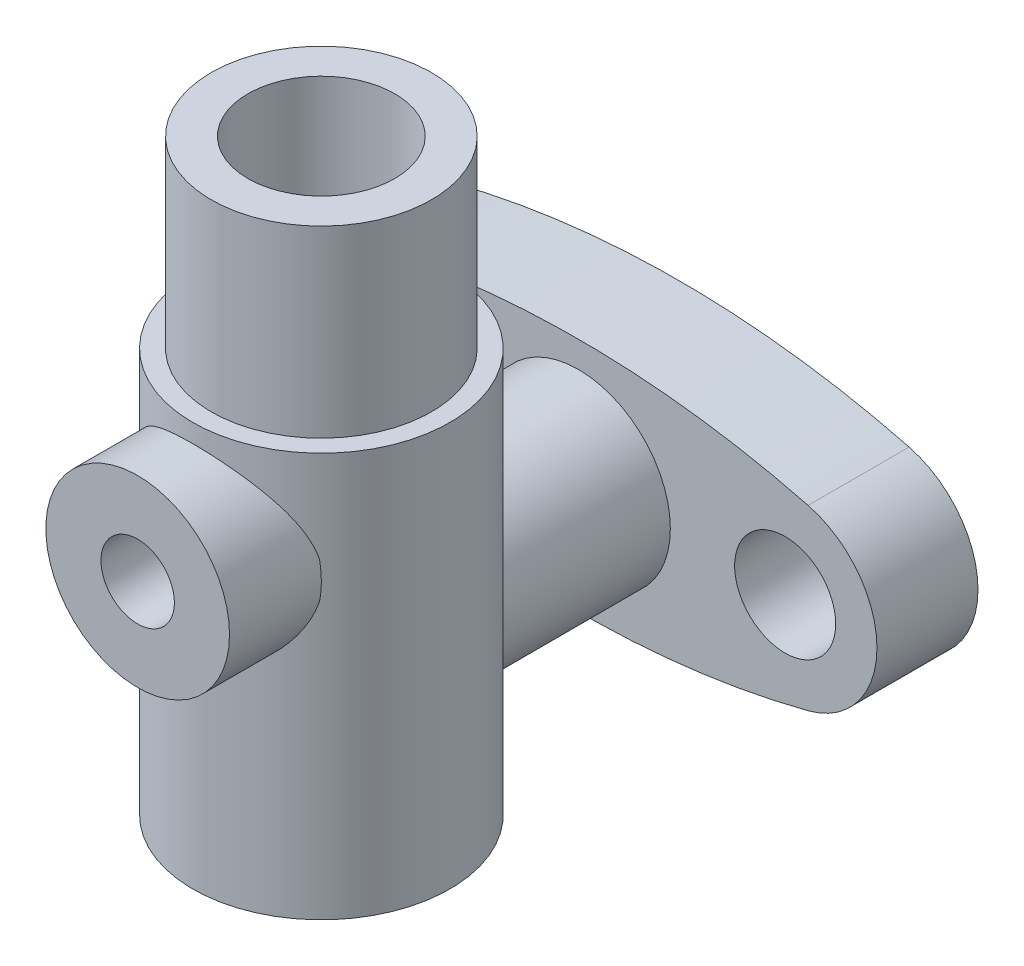
SolidWorks part; units mm, degrees
material "Plain Carbon Steel"
ref_plane "Front Plane" through (0, 0, 0) normal (0, 0, 1) x (1, 0, 0)
ref_plane "Top Plane" through (0, 0, 0) normal (0, 1, 0) x (1, 0, 0)
ref_plane "Right Plane" through (0, 0, 0) normal (1, 0, 0) x (0, 0, -1)
sketch "Main Body Profile Sketch" plane through (0, 0, 0) normal (0, 0, 1) x (1, 0, 0)
  line L0 (0, 64) -> (0, 0) construction
  line L1 (0, 64) -> (12, 64)
  line L2 (12, 64) -> (12, 44)
  line L3 (12, 44) -> (14, 44)
  line L4 (14, 44) -> (14, 0)
  line L5 (14, 0) -> (0, 0)
  line L6 (0, 0) -> (0, 64)
  dimension "D1" = 24
  dimension "D2" = 28
  dimension "D3" = 64
  dimension "D4" = 44
revolve "Main Body Revolve" add sketch "Main Body Profile Sketch" angle 360 about L0
cosmetic thread "Cosmetic Thread1" parameters "D1"=19, "D2"=13.797
ref_plane "Plane1" through (0, 0, 20) normal (0, 0, 1) x (1, 0, 0)
sketch "Side Port Boss Sketch" plane through (0, 0, 20) normal (0, 0, 1) x (1, 0, 0)
  circle A0 centre (0, 32) radius 10
  dimension "D1" = 20
  dimension "D2" = 32
extrude "Side Port Boss" add sketch "Side Port Boss Sketch" against normal blind 10 from surface at 0 starting at plane "Plane1"
ref_plane "Plane2" through (0, 0, -39) normal (0, 0, 1) x (1, 0, 0)
sketch "Mounting Ear Sketch" plane through (0, 0, -39) normal (0, 0, 1) x (1, 0, 0)
  line L0 (0, 0) -> (0, 64) construction
  line L1 (12, 64) -> (-12, 64) construction
  circle A0 centre (0, 18) radius 4
  arc A1 (-25, 27.6825) -> (-25, 8.3175) centre (-22.5, 18) ccw
  circle A3 centre (-22.5, 18) radius 5.5
  circle A4 centre (22.5, 18) radius 5.5
  arc A5 (25, 27.6825) -> (25, 8.3175) centre (22.5, 18) cw
  arc A6 (-25, 27.6825) -> (25, 27.6825) centre (0, -69.1421) cw
  arc A7 (-25, 8.3175) -> (25, 8.3175) centre (0, 105.1421) ccw
  dimension "D1" = 20
  dimension "D2" = 11
  dimension "D3" = 8
  dimension "D7" = 100
  dimension "D8" = 100
  dimension "D4" = 18
  dimension "D5" = 22.5
  dimension "D6" = 18
extrude "Mounting Ear" add sketch "Mounting Ear Sketch" along normal blind 11 separate body contours L0 A7 A5 A6 A0 A4 | A7 L0 A0 A6 A1 A3 | A0 L0 | L0 A0
sketch "Ear Hub Sketch" plane through (0, 0, -28) normal (0, 0, 1) x (1, 0, 0)
  circle A0 centre (0, 18) radius 10
  dimension "D1" = 20
  dimension "D2" = 18
extrude "Ear Hub Boss" add sketch "Ear Hub Sketch" along normal up to surface (18.202 mm away)
sketch "Bore Profile Sketch" plane through (0, 0, 0) normal (1, 0, 0) x (0, 0, -1)
  line L0 (0, 64) -> (0, 0) construction
  line L1 (12, 64) -> (-12, 64) construction
  line L2 (0, 64) -> (8, 64)
  line L3 (8, 64) -> (8, 49)
  line L4 (8, 49) -> (4, 46.6906)
  line L5 (4, 46.6906) -> (4, 33.7321)
  line L6 (4, 33.7321) -> (5, 32)
  line L7 (5, 32) -> (5, 28.9282)
  line L8 (5, 28.9282) -> (9, 22)
  line L9 (9, 22) -> (9, 12)
  line L10 (9, 12) -> (8, 12)
  line L11 (8, 12) -> (8, 0)
  line L12 (-14, 0) -> (14, 0) construction
  line L13 (8, 0) -> (0, 0)
  line L14 (14, 44) -> (-14, 44) construction
  line L15 (0, 64) -> (0, 0)
  dimension "D1" = 16
  dimension "D2" = 16
  dimension "D3" = 18
  dimension "D4" = 10
  dimension "D5" = 8
  dimension "D6" = 60
  dimension "D7" = 15
  dimension "D8" = 12
  dimension "D9" = 22
  dimension "D10" = 12
revolve "Bore Revolve Cut" cut sketch "Bore Profile Sketch" angle 360 about L0
hole_wizard "Ear Hole Ø8" positions "Sketch10" profile "Sketch11" hole size "Ø8.0" standard "ANSI Metric"
sketch "Sketch10" plane through (0, 0, -39) normal (0, 0, -1) x (-1, 0, 0)
  point P0 (0, 18)
sketch "Sketch11" plane through (0, 18, -39) normal (1, 0, 0) x (0, 1, 0)
  line L0 (0, 0) -> (0, 33.3564)
  line L1 (0, 33.3564) -> (4, 30)
  line L2 (4, 30) -> (4, 0)
  line L5 (4, 0) -> (0, 0)
  line L10 (0, 33.3564) -> (-4, 30) construction
  line L11 (0, -6.35) -> (0, 107.95) construction
  dimension "Hole Dia." = 8
  dimension "Hole Depth" = 30
  dimension "Drill Angle" = 100
hole_wizard "Side Port Tapped Hole M8x1.0" positions "Sketch12" profile "Sketch13" tap size "M8x1.0" standard "ANSI Metric"
sketch "Sketch12" plane through (0, 0, 20) normal (0, 0, 1) x (1, 0, 0)
  point P0 (0, 32)
sketch "Sketch13" plane through (0, 32, 20) normal (1, 0, 0) x (0, -1, 0)
  line L0 (0, 0) -> (0, 20)
  line L1 (0, 20) -> (4, 17.5966)
  line L2 (4, 17.5966) -> (4, 0)
  line L5 (4, 0) -> (0, 0)
  line L10 (0, 20) -> (-4, 17.5966) construction
  line L11 (0, -6.35) -> (0, 107.95) construction
  dimension "Tap Drill Dia." = 8
  dimension "Tap Drill Depth" = 20
  dimension "Drill Angle" = 118
cosmetic thread "Hole Thread1" parameters "D1"=16, "D2"=8
